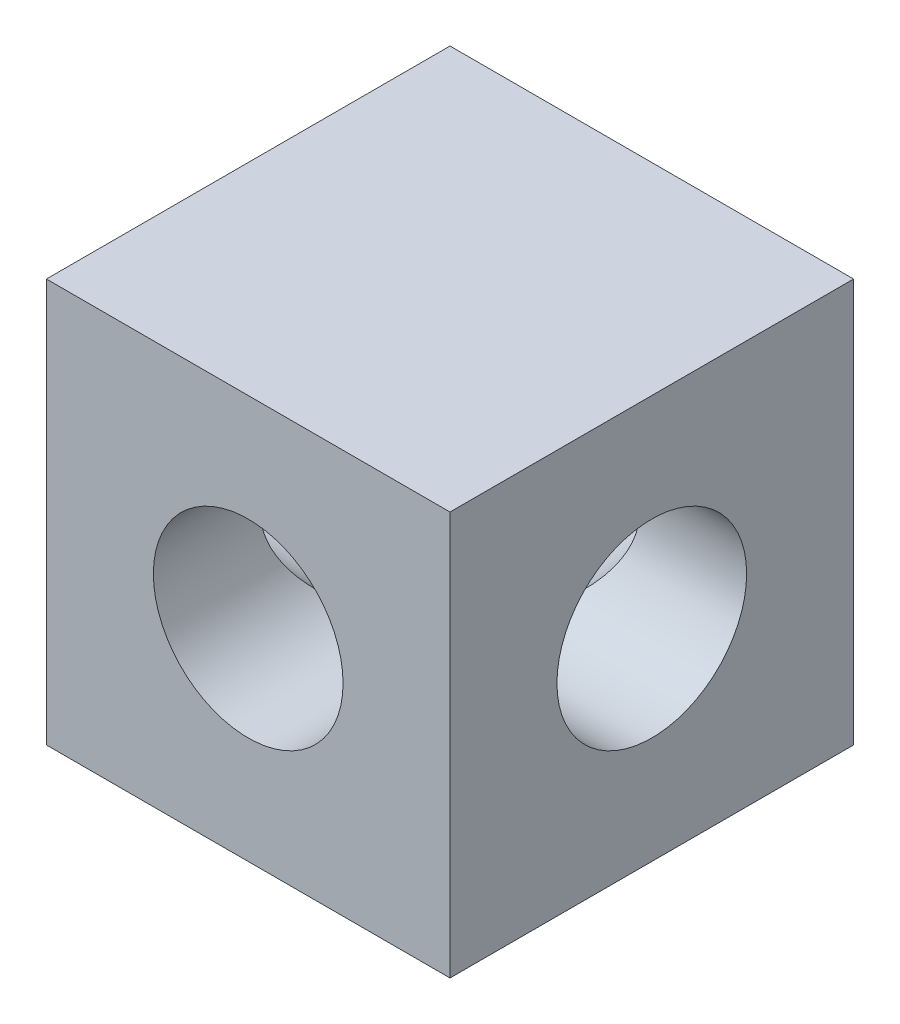
ISO-10303-21;
HEADER;
FILE_DESCRIPTION(('STEP AP214'),'2;1');
FILE_NAME('part.step','',(''),(''),'','','');
FILE_SCHEMA(('AUTOMOTIVE_DESIGN { 1 0 10303 214 1 1 1 1 }'));
ENDSEC;
DATA;
#1=APPLICATION_CONTEXT('core data for automotive mechanical design processes');
#2=APPLICATION_PROTOCOL_DEFINITION('international standard','automotive_design',2000,#1);
#3=PRODUCT_CONTEXT('',#1,'mechanical');
#4=PRODUCT('Part','Part','',(#3));
#5=PRODUCT_RELATED_PRODUCT_CATEGORY('part','',(#4));
#6=PRODUCT_DEFINITION_FORMATION('','',#4);
#7=PRODUCT_DEFINITION_CONTEXT('part definition',#1,'design');
#8=PRODUCT_DEFINITION('design','',#6,#7);
#9=PRODUCT_DEFINITION_SHAPE('','',#8);
#10=(LENGTH_UNIT() NAMED_UNIT(*) SI_UNIT(.MILLI.,.METRE.));
#11=(NAMED_UNIT(*) PLANE_ANGLE_UNIT() SI_UNIT($,.RADIAN.));
#12=(NAMED_UNIT(*) SI_UNIT($,.STERADIAN.) SOLID_ANGLE_UNIT());
#13=UNCERTAINTY_MEASURE_WITH_UNIT(LENGTH_MEASURE(1.E-05),#10,'distance_accuracy_value','');
#14=(GEOMETRIC_REPRESENTATION_CONTEXT(3) GLOBAL_UNCERTAINTY_ASSIGNED_CONTEXT((#13)) GLOBAL_UNIT_ASSIGNED_CONTEXT((#10,
#11,#12)) REPRESENTATION_CONTEXT('',''));
#15=CARTESIAN_POINT('',(0.,0.,0.));
#16=DIRECTION('',(0.,0.,1.));
#17=DIRECTION('',(1.,0.,0.));
#18=AXIS2_PLACEMENT_3D('',#15,#16,#17);
#19=CARTESIAN_POINT('',(0.,10.16,-10.16));
#20=DIRECTION('',(0.,0.,1.));
#21=DIRECTION('',(1.,0.,0.));
#22=AXIS2_PLACEMENT_3D('',#19,#20,#21);
#23=CYLINDRICAL_SURFACE('',#22,4.775);
#24=CARTESIAN_POINT('',(0.,10.16,10.16));
#25=DIRECTION('',(0.,0.,1.));
#26=DIRECTION('',(1.,0.,0.));
#27=AXIS2_PLACEMENT_3D('',#24,#25,#26);
#28=CIRCLE('',#27,4.775);
#29=CARTESIAN_POINT('',(4.775,10.16,10.16));
#30=VERTEX_POINT('',#29);
#31=EDGE_CURVE('E132',#30,#30,#28,.T.);
#32=ORIENTED_EDGE('',*,*,#31,.T.);
#33=EDGE_LOOP('',(#32));
#34=FACE_BOUND('',#33,.T.);
#35=CARTESIAN_POINT('',(0.,10.16,0.));
#36=DIRECTION('',(-0.707106781186547,0.,0.707106781186548));
#37=DIRECTION('',(0.707106781186548,0.,0.707106781186547));
#38=AXIS2_PLACEMENT_3D('',#35,#36,#37);
#39=ELLIPSE('',#38,6.75286976033153,4.775);
#40=CARTESIAN_POINT('',(0.,14.935,0.));
#41=VERTEX_POINT('',#40);
#42=CARTESIAN_POINT('',(0.,5.385,0.));
#43=VERTEX_POINT('',#42);
#44=EDGE_CURVE('E55',#41,#43,#39,.F.);
#45=ORIENTED_EDGE('',*,*,#44,.T.);
#46=CARTESIAN_POINT('',(0.,10.16,0.));
#47=DIRECTION('',(0.707106781186548,0.,0.707106781186547));
#48=DIRECTION('',(-0.707106781186547,0.,0.707106781186548));
#49=AXIS2_PLACEMENT_3D('',#46,#47,#48);
#50=ELLIPSE('',#49,6.75286976033153,4.775);
#51=EDGE_CURVE('E11',#43,#41,#50,.F.);
#52=ORIENTED_EDGE('',*,*,#51,.T.);
#53=EDGE_LOOP('',(#45,#52));
#54=FACE_BOUND('',#53,.T.);
#55=ADVANCED_FACE('F39',(#34,#54),#23,.F.);
#56=CARTESIAN_POINT('',(10.16,20.32,-10.16));
#57=DIRECTION('',(-1.,0.,0.));
#58=DIRECTION('',(0.,0.,1.));
#59=AXIS2_PLACEMENT_3D('',#56,#57,#58);
#60=PLANE('',#59);
#61=CARTESIAN_POINT('',(10.16,10.16,0.));
#62=DIRECTION('',(1.,0.,0.));
#63=DIRECTION('',(0.,0.,-1.));
#64=AXIS2_PLACEMENT_3D('',#61,#62,#63);
#65=CIRCLE('',#64,4.775);
#66=CARTESIAN_POINT('',(10.16,10.16,-4.775));
#67=VERTEX_POINT('',#66);
#68=EDGE_CURVE('E137',#67,#67,#65,.T.);
#69=ORIENTED_EDGE('',*,*,#68,.F.);
#70=EDGE_LOOP('',(#69));
#71=FACE_BOUND('',#70,.T.);
#72=DIRECTION('',(0.,0.,-1.));
#73=VECTOR('',#72,1.);
#74=CARTESIAN_POINT('',(10.16,0.,-10.16));
#75=LINE('',#74,#73);
#76=CARTESIAN_POINT('',(10.16,0.,10.16));
#77=VERTEX_POINT('',#76);
#78=CARTESIAN_POINT('',(10.16,0.,-10.16));
#79=VERTEX_POINT('',#78);
#80=EDGE_CURVE('E122',#77,#79,#75,.T.);
#81=ORIENTED_EDGE('',*,*,#80,.T.);
#82=DIRECTION('',(0.,-1.,0.));
#83=VECTOR('',#82,1.);
#84=CARTESIAN_POINT('',(10.16,20.32,-10.16));
#85=LINE('',#84,#83);
#86=CARTESIAN_POINT('',(10.16,20.32,-10.16));
#87=VERTEX_POINT('',#86);
#88=EDGE_CURVE('E103',#87,#79,#85,.T.);
#89=ORIENTED_EDGE('',*,*,#88,.F.);
#90=DIRECTION('',(0.,0.,-1.));
#91=VECTOR('',#90,1.);
#92=CARTESIAN_POINT('',(10.16,20.32,-10.16));
#93=LINE('',#92,#91);
#94=CARTESIAN_POINT('',(10.16,20.32,10.16));
#95=VERTEX_POINT('',#94);
#96=EDGE_CURVE('E119',#95,#87,#93,.T.);
#97=ORIENTED_EDGE('',*,*,#96,.F.);
#98=DIRECTION('',(0.,-1.,0.));
#99=VECTOR('',#98,1.);
#100=CARTESIAN_POINT('',(10.16,20.32,10.16));
#101=LINE('',#100,#99);
#102=EDGE_CURVE('E111',#95,#77,#101,.T.);
#103=ORIENTED_EDGE('',*,*,#102,.T.);
#104=EDGE_LOOP('',(#81,#89,#97,#103));
#105=FACE_BOUND('',#104,.T.);
#106=ADVANCED_FACE('F41',(#71,#105),#60,.F.);
#107=CARTESIAN_POINT('',(-10.16,20.32,-10.16));
#108=DIRECTION('',(0.,0.,1.));
#109=DIRECTION('',(1.,0.,0.));
#110=AXIS2_PLACEMENT_3D('',#107,#108,#109);
#111=PLANE('',#110);
#112=CARTESIAN_POINT('',(0.,10.16,-10.16));
#113=DIRECTION('',(0.,0.,1.));
#114=DIRECTION('',(1.,0.,0.));
#115=AXIS2_PLACEMENT_3D('',#112,#113,#114);
#116=CIRCLE('',#115,4.775);
#117=CARTESIAN_POINT('',(4.775,10.16,-10.16));
#118=VERTEX_POINT('',#117);
#119=EDGE_CURVE('E125',#118,#118,#116,.T.);
#120=ORIENTED_EDGE('',*,*,#119,.T.);
#121=EDGE_LOOP('',(#120));
#122=FACE_BOUND('',#121,.T.);
#123=DIRECTION('',(-1.,0.,0.));
#124=VECTOR('',#123,1.);
#125=CARTESIAN_POINT('',(-10.16,0.,-10.16));
#126=LINE('',#125,#124);
#127=CARTESIAN_POINT('',(-10.16,0.,-10.16));
#128=VERTEX_POINT('',#127);
#129=EDGE_CURVE('E118',#79,#128,#126,.T.);
#130=ORIENTED_EDGE('',*,*,#129,.T.);
#131=DIRECTION('',(0.,-1.,0.));
#132=VECTOR('',#131,1.);
#133=CARTESIAN_POINT('',(-10.16,20.32,-10.16));
#134=LINE('',#133,#132);
#135=CARTESIAN_POINT('',(-10.16,20.32,-10.16));
#136=VERTEX_POINT('',#135);
#137=EDGE_CURVE('E108',#136,#128,#134,.T.);
#138=ORIENTED_EDGE('',*,*,#137,.F.);
#139=DIRECTION('',(-1.,0.,0.));
#140=VECTOR('',#139,1.);
#141=CARTESIAN_POINT('',(-10.16,20.32,-10.16));
#142=LINE('',#141,#140);
#143=EDGE_CURVE('E89',#87,#136,#142,.T.);
#144=ORIENTED_EDGE('',*,*,#143,.F.);
#145=ORIENTED_EDGE('',*,*,#88,.T.);
#146=EDGE_LOOP('',(#130,#138,#144,#145));
#147=FACE_BOUND('',#146,.T.);
#148=ADVANCED_FACE('F157',(#122,#147),#111,.F.);
#149=CARTESIAN_POINT('',(-10.16,20.32,-10.16));
#150=DIRECTION('',(1.,0.,0.));
#151=DIRECTION('',(0.,0.,-1.));
#152=AXIS2_PLACEMENT_3D('',#149,#150,#151);
#153=PLANE('',#152);
#154=CARTESIAN_POINT('',(-10.16,10.16,0.));
#155=DIRECTION('',(1.,0.,0.));
#156=DIRECTION('',(0.,0.,-1.));
#157=AXIS2_PLACEMENT_3D('',#154,#155,#156);
#158=CIRCLE('',#157,4.775);
#159=CARTESIAN_POINT('',(-10.16,10.16,-4.775));
#160=VERTEX_POINT('',#159);
#161=EDGE_CURVE('E131',#160,#160,#158,.T.);
#162=ORIENTED_EDGE('',*,*,#161,.T.);
#163=EDGE_LOOP('',(#162));
#164=FACE_BOUND('',#163,.T.);
#165=DIRECTION('',(0.,0.,1.));
#166=VECTOR('',#165,1.);
#167=CARTESIAN_POINT('',(-10.16,0.,-10.16));
#168=LINE('',#167,#166);
#169=CARTESIAN_POINT('',(-10.16,0.,10.16));
#170=VERTEX_POINT('',#169);
#171=EDGE_CURVE('E120',#128,#170,#168,.T.);
#172=ORIENTED_EDGE('',*,*,#171,.T.);
#173=DIRECTION('',(0.,-1.,0.));
#174=VECTOR('',#173,1.);
#175=CARTESIAN_POINT('',(-10.16,20.32,10.16));
#176=LINE('',#175,#174);
#177=CARTESIAN_POINT('',(-10.16,20.32,10.16));
#178=VERTEX_POINT('',#177);
#179=EDGE_CURVE('E115',#178,#170,#176,.T.);
#180=ORIENTED_EDGE('',*,*,#179,.F.);
#181=DIRECTION('',(0.,0.,1.));
#182=VECTOR('',#181,1.);
#183=CARTESIAN_POINT('',(-10.16,20.32,-10.16));
#184=LINE('',#183,#182);
#185=EDGE_CURVE('E130',#136,#178,#184,.T.);
#186=ORIENTED_EDGE('',*,*,#185,.F.);
#187=ORIENTED_EDGE('',*,*,#137,.T.);
#188=EDGE_LOOP('',(#172,#180,#186,#187));
#189=FACE_BOUND('',#188,.T.);
#190=ADVANCED_FACE('F141',(#164,#189),#153,.F.);
#191=CARTESIAN_POINT('',(-10.16,20.32,10.16));
#192=DIRECTION('',(0.,0.,-1.));
#193=DIRECTION('',(-1.,0.,0.));
#194=AXIS2_PLACEMENT_3D('',#191,#192,#193);
#195=PLANE('',#194);
#196=ORIENTED_EDGE('',*,*,#31,.F.);
#197=EDGE_LOOP('',(#196));
#198=FACE_BOUND('',#197,.T.);
#199=DIRECTION('',(1.,0.,0.));
#200=VECTOR('',#199,1.);
#201=CARTESIAN_POINT('',(-10.16,0.,10.16));
#202=LINE('',#201,#200);
#203=EDGE_CURVE('E82',#170,#77,#202,.T.);
#204=ORIENTED_EDGE('',*,*,#203,.T.);
#205=ORIENTED_EDGE('',*,*,#102,.F.);
#206=DIRECTION('',(1.,0.,0.));
#207=VECTOR('',#206,1.);
#208=CARTESIAN_POINT('',(-10.16,20.32,10.16));
#209=LINE('',#208,#207);
#210=EDGE_CURVE('E62',#178,#95,#209,.T.);
#211=ORIENTED_EDGE('',*,*,#210,.F.);
#212=ORIENTED_EDGE('',*,*,#179,.T.);
#213=EDGE_LOOP('',(#204,#205,#211,#212));
#214=FACE_BOUND('',#213,.T.);
#215=ADVANCED_FACE('F173',(#198,#214),#195,.F.);
#216=CARTESIAN_POINT('',(0.,20.32,0.));
#217=DIRECTION('',(0.,1.,0.));
#218=DIRECTION('',(0.,0.,1.));
#219=AXIS2_PLACEMENT_3D('',#216,#217,#218);
#220=PLANE('',#219);
#221=ORIENTED_EDGE('',*,*,#96,.T.);
#222=ORIENTED_EDGE('',*,*,#143,.T.);
#223=ORIENTED_EDGE('',*,*,#185,.T.);
#224=ORIENTED_EDGE('',*,*,#210,.T.);
#225=EDGE_LOOP('',(#221,#222,#223,#224));
#226=FACE_BOUND('',#225,.T.);
#227=ADVANCED_FACE('F169',(#226),#220,.T.);
#228=CARTESIAN_POINT('',(0.,0.,0.));
#229=DIRECTION('',(0.,1.,0.));
#230=DIRECTION('',(0.,0.,1.));
#231=AXIS2_PLACEMENT_3D('',#228,#229,#230);
#232=PLANE('',#231);
#233=ORIENTED_EDGE('',*,*,#80,.F.);
#234=ORIENTED_EDGE('',*,*,#203,.F.);
#235=ORIENTED_EDGE('',*,*,#171,.F.);
#236=ORIENTED_EDGE('',*,*,#129,.F.);
#237=EDGE_LOOP('',(#233,#234,#235,#236));
#238=FACE_BOUND('',#237,.T.);
#239=ADVANCED_FACE('F162',(#238),#232,.F.);
#240=CARTESIAN_POINT('',(0.,10.16,0.));
#241=DIRECTION('',(-0.707106781186547,0.,0.707106781186548));
#242=DIRECTION('',(0.707106781186548,0.,0.707106781186547));
#243=AXIS2_PLACEMENT_3D('',#240,#241,#242);
#244=ELLIPSE('',#243,6.75286976033153,4.775);
#245=EDGE_CURVE('E96',#41,#43,#244,.T.);
#246=ORIENTED_EDGE('',*,*,#245,.T.);
#247=CARTESIAN_POINT('',(0.,10.16,0.));
#248=DIRECTION('',(0.707106781186548,0.,0.707106781186547));
#249=DIRECTION('',(-0.707106781186547,0.,0.707106781186548));
#250=AXIS2_PLACEMENT_3D('',#247,#248,#249);
#251=ELLIPSE('',#250,6.75286976033153,4.775);
#252=EDGE_CURVE('E50',#43,#41,#251,.T.);
#253=ORIENTED_EDGE('',*,*,#252,.T.);
#254=EDGE_LOOP('',(#246,#253));
#255=FACE_BOUND('',#254,.T.);
#256=ORIENTED_EDGE('',*,*,#119,.F.);
#257=EDGE_LOOP('',(#256));
#258=FACE_BOUND('',#257,.T.);
#259=ADVANCED_FACE('F104',(#255,#258),#23,.F.);
#260=CARTESIAN_POINT('',(-10.16,10.16,0.));
#261=DIRECTION('',(1.,0.,0.));
#262=DIRECTION('',(0.,0.,-1.));
#263=AXIS2_PLACEMENT_3D('',#260,#261,#262);
#264=CYLINDRICAL_SURFACE('',#263,4.775);
#265=ORIENTED_EDGE('',*,*,#68,.T.);
#266=EDGE_LOOP('',(#265));
#267=FACE_BOUND('',#266,.T.);
#268=ORIENTED_EDGE('',*,*,#44,.F.);
#269=ORIENTED_EDGE('',*,*,#252,.F.);
#270=EDGE_LOOP('',(#268,#269));
#271=FACE_BOUND('',#270,.T.);
#272=ADVANCED_FACE('F105',(#267,#271),#264,.F.);
#273=ORIENTED_EDGE('',*,*,#161,.F.);
#274=EDGE_LOOP('',(#273));
#275=FACE_BOUND('',#274,.T.);
#276=ORIENTED_EDGE('',*,*,#245,.F.);
#277=ORIENTED_EDGE('',*,*,#51,.F.);
#278=EDGE_LOOP('',(#276,#277));
#279=FACE_BOUND('',#278,.T.);
#280=ADVANCED_FACE('F100',(#275,#279),#264,.F.);
#281=CLOSED_SHELL('',(#55,#106,#148,#190,#215,#227,#239,#259,#272,#280));
#282=MANIFOLD_SOLID_BREP('B2',#281);
#283=ADVANCED_BREP_SHAPE_REPRESENTATION('',(#18,#282),#14);
#284=SHAPE_DEFINITION_REPRESENTATION(#9,#283);
ENDSEC;
END-ISO-10303-21;
